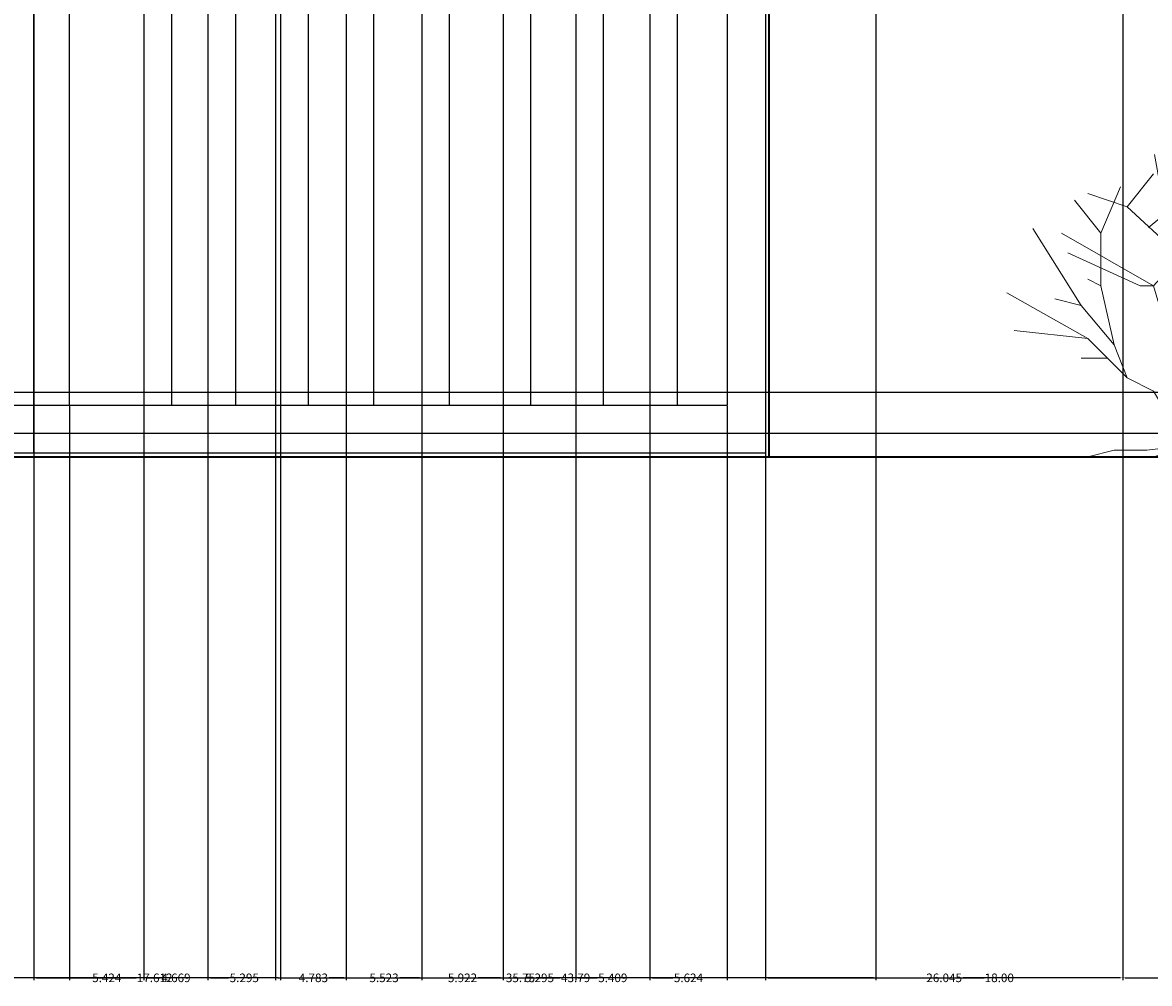
# Model space of a CAD drawing. Units: inches. Extents: x -13 to 809, y 112 to 656.
# Tile 11 of 55: x 257 to 339, y 112 to 182. Entities that reach past the tile are written whole.
import ezdxf

# ---------------------------------------------------------------- set-up
doc = ezdxf.new("R2010")
doc.units = ezdxf.units.IN
doc.header["$MEASUREMENT"] = 0
for name, color, linetype, lineweight in [('A-ANNO-DIMS', 2, 'Continuous', 18), ('A-DOOR', 4, 'Continuous', 25), ('A-ELEV', 7, 'Continuous', 35), ('L-PLNT', 3, 'Continuous', 18)]:
    doc.layers.add(name, color=color, linetype=linetype, lineweight=lineweight)
doc.styles.get("Standard").update_dxf_attribs({"font": 'arial.ttf'})
doc.dimstyles.get("Standard").update_dxf_attribs({"dimtxt": 0.625, "dimasz": 0.18, "dimexe": 0.18, "dimexo": 0.0625, "dimgap": 0.09, "dimtad": 0, "dimtih": 1, "dimtoh": 1, "dimdec": 4, "dimzin": 0, "dimdsep": 46, "dimlunit": 4, "dimtxsty": 'Standard', "dimcen": 0.09, "dimadec": 0, "dimazin": 0, "dimtfac": 1, "dimtdec": 4, "dimtofl": 0, "dimtmove": 0, "dimatfit": 3, "dimfxl": 1, "dimtolj": 1, "dimtzin": 0, "dimarcsym": 0})

# ---------------------------------------------------------------- blocks, each defined once
blk = doc.blocks.new('Shrub - elevation')
for p, q in [((-11.433, 18.289), (-10.457, 22.749)), ((-9.48, 19.775), (-8.992, 22.592)), ((-12.471, 19.775), (-12.898, 22.044)), ((-8.16, 17.76), (-10.56, 21.6)), ((-5.28, 19.2), (-3.84, 21.6)), ((-3.377, 18.602), (-2.888, 21.575)), ((-0.508, 21.888), (-0.081, 20.558)), ((0.041, 20.714), (1.384, 22.044)), ((0.102, 21.34), (0.835, 21.888)), ((-14.88, 18.24), (-12.96, 20.64)), ((-11.28, 19.619), (-12.104, 21.184)), ((-7.2, 19.68), (-6.24, 21.12)), ((-5.086, 17.741), (-5.513, 21.34)), ((-3.84, 16.8), (-0.96, 20.64)), ((-0.203, 19.149), (0.102, 21.34)), ((-0.02, 20.01), (0.896, 21.105)), ((-11.677, 19.071), (-12.471, 19.775)), ((-11.921, 18.836), (-10.64, 20.401)), ((-7.2, 19.68), (-8.64, 20.16)), ((-2.88, 15.84), (-2.4, 20.16)), ((-0.142, 19.384), (0.59, 20.401)), ((-14.88, 18.24), (-17.76, 19.2)), ((-16.8, 16.32), (-15.36, 19.68)), ((-10.579, 18.054), (-9.846, 19.697)), ((-8.16, 17.76), (-5.28, 19.2)), ((-4.8, 16.32), (-7.2, 19.68)), ((-2.88, 12.96), (-4.32, 19.68)), ((0.346, 13.203), (-0.203, 19.149)), ((-16.8, 16.32), (-18.72, 18.72)), ((-8.16, 12), (-14.88, 18.24)), ((-13.325, 16.724), (-11.433, 18.289)), ((-12.043, 15.628), (-11.921, 18.836)), ((-2.766, 16.802), (-3.377, 18.602)), ((1.323, 16.254), (3.642, 18.289)), ((-12.96, 12.48), (-8.16, 17.76)), ((-11.982, 16.802), (-10.579, 18.054)), ((-3.377, 15.315), (-5.086, 17.819)), ((1.44, 15.36), (2.88, 17.28)), ((-18.24, 11.04), (-21.755, 16.655)), ((-7.2, 14.88), (-3.84, 16.8)), ((-12.96, 12.48), (-19.68, 16.32)), ((-16.8, 12.48), (-16.8, 16.32)), ((-0.96, 10.56), (-2.88, 15.84)), ((0.346, 13.203), (1.323, 16.254)), ((2.4, 15.36), (3.36, 16.32)), ((-13.92, 12.48), (-19.2, 14.88)), ((-7.68, 12.48), (-7.2, 14.88)), ((0.96, 12), (1.44, 15.36)), ((0.96, 12), (2.88, 14.88)), ((1.92, 13.44), (2.4, 15.36)), ((-0.48, 10.8), (0.346, 13.203)), ((-16.8, 12.48), (-17.76, 12.96)), ((-15.84, 8.16), (-16.8, 12.48)), ((-12.96, 12.48), (-13.92, 12.48)), ((-10.56, 4.32), (-12.96, 12.48)), ((-6.72, 8.64), (-7.68, 12.48)), ((-3.36, 5.28), (-2.88, 12.96)), ((-17.76, 8.64), (-23.663, 11.961)), ((-18.24, 11.04), (-20.16, 11.52)), ((-8.64, 7.68), (-8.16, 12)), ((-1.92, 9.6), (0.96, 12)), ((-15.84, 8.16), (-18.24, 11.04)), ((-17.76, 8.64), (-23.128, 9.222)), ((-4.32, 2.88), (-1.92, 9.6)), ((-14.88, 5.76), (-17.76, 8.64)), ((-5.76, 5.28), (-6.72, 8.64)), ((-14.88, 5.76), (-15.84, 8.16)), ((-10.56, 4.32), (-8.64, 7.68)), ((-16.32, 7.2), (-18.24, 7.2)), ((-12.96, 4.8), (-14.88, 5.76)), ((-6.24, 2.88), (-5.76, 5.28)), ((-11.52, 2.4), (-12.96, 4.8)), ((-8.64, 1.92), (-10.56, 4.32)), ((-8.64, 0.96), (-4.32, 2.88)), ((-8.64, 0.96), (-6.24, 2.88)), ((-8.64, 0.96), (-11.52, 2.4)), ((-8.64, 0.96), (-8.64, 1.92)), ((-9.6, 0.96), (-13.44, 0.48)), ((-9.6, 0.96), (-12.96, 0)), ((-9.6, 0.96), (-7.68, 0.96)), ((-8.64, 0.96), (-2.88, 0.96)), ((-7.68, 0.96), (-6.24, 0.48)), ((-2.88, 0.96), (0, 0)), ((-15.84, 0.48), (-17.76, 0)), ((-13.44, 0.48), (-15.84, 0.48)), ((-6.24, 0.48), (-3.36, 0))]:
    blk.add_line(p, q)
blk = doc.blocks.new('*D15')
at = {"layer": 'A-ANNO-DIMS', "color": 0, "lineweight": -2, "transparency": 16777216}
for p, q in [((210.079, 223.038), (210.079, 112.34)), ((258.102, 210.722), (258.102, 112.34)), ((210.259, 112.52), (232.937, 112.52)), ((257.922, 112.52), (235.245, 112.52))]:
    blk.add_line(p, q, dxfattribs=at)
at = {"layer": 'A-ANNO-DIMS', "color": 0, "transparency": 16777216}
for points in [[(210.259, 112.55), (210.259, 112.49), (210.079, 112.52)], [(257.922, 112.55), (257.922, 112.49), (258.102, 112.52)]]:
    blk.add_solid(points, dxfattribs=at)
at = {"layer": 'Defpoints', "color": 0, "transparency": 16777216}
for p in [(210.079, 223.1), (258.102, 210.785), (258.102, 112.52)]:
    blk.add_point(p, dxfattribs=at)
at = {"layer": 'A-ANNO-DIMS', "color": 0, "transparency": 16777216, "insert": (234.091, 112.52), "char_height": 0.625, "attachment_point": 5}
blk.add_mtext('\\A1;48.02', dxfattribs=at)
blk = doc.blocks.new('*D16')
at = {"layer": 'A-ANNO-DIMS', "color": 0, "lineweight": -2, "transparency": 16777216}
for p, q in [((275.715, 223.038), (275.715, 112.34)), ((258.102, 210.722), (258.102, 112.34)), ((258.282, 112.52), (265.554, 112.52)), ((275.535, 112.52), (268.263, 112.52))]:
    blk.add_line(p, q, dxfattribs=at)
at = {"layer": 'A-ANNO-DIMS', "color": 0, "transparency": 16777216}
for points in [[(258.282, 112.55), (258.282, 112.49), (258.102, 112.52)], [(275.535, 112.55), (275.535, 112.49), (275.715, 112.52)]]:
    blk.add_solid(points, dxfattribs=at)
at = {"layer": 'Defpoints', "color": 0, "transparency": 16777216}
for p in [(275.715, 223.1), (258.102, 210.785), (275.715, 112.52)]:
    blk.add_point(p, dxfattribs=at)
at = {"layer": 'A-ANNO-DIMS', "color": 0, "transparency": 16777216, "insert": (266.908, 112.52), "char_height": 0.625, "attachment_point": 5}
blk.add_mtext('\\A1;17.612', dxfattribs=at)
blk = doc.blocks.new('*D17')
at = {"layer": 'A-ANNO-DIMS', "color": 0, "lineweight": -2, "transparency": 16777216}
for p, q in [((275.715, 223.038), (275.715, 112.34)), ((311.463, 210.722), (311.463, 112.34)), ((275.895, 112.52), (292.442, 112.52)), ((311.283, 112.52), (294.735, 112.52))]:
    blk.add_line(p, q, dxfattribs=at)
at = {"layer": 'A-ANNO-DIMS', "color": 0, "transparency": 16777216}
for points in [[(275.895, 112.55), (275.895, 112.49), (275.715, 112.52)], [(311.283, 112.55), (311.283, 112.49), (311.463, 112.52)]]:
    blk.add_solid(points, dxfattribs=at)
at = {"layer": 'Defpoints', "color": 0, "transparency": 16777216}
for p in [(275.715, 223.1), (311.463, 210.785), (311.463, 112.52)]:
    blk.add_point(p, dxfattribs=at)
at = {"layer": 'A-ANNO-DIMS', "color": 0, "transparency": 16777216, "insert": (293.589, 112.52), "char_height": 0.625, "attachment_point": 5}
blk.add_mtext('\\A1;35.75', dxfattribs=at)
blk = doc.blocks.new('*D18')
at = {"layer": 'A-ANNO-DIMS', "color": 0, "lineweight": -2, "transparency": 16777216}
for p, q in [((337.507, 306.457), (337.507, 112.34)), ((311.463, 210.722), (311.463, 112.34)), ((311.643, 112.52), (323.09, 112.52)), ((337.327, 112.52), (325.88, 112.52))]:
    blk.add_line(p, q, dxfattribs=at)
at = {"layer": 'A-ANNO-DIMS', "color": 0, "transparency": 16777216}
for points in [[(311.643, 112.55), (311.643, 112.49), (311.463, 112.52)], [(337.327, 112.55), (337.327, 112.49), (337.507, 112.52)]]:
    blk.add_solid(points, dxfattribs=at)
at = {"layer": 'Defpoints', "color": 0, "transparency": 16777216}
for p in [(337.507, 306.52), (311.463, 210.785), (337.507, 112.52)]:
    blk.add_point(p, dxfattribs=at)
at = {"layer": 'A-ANNO-DIMS', "color": 0, "transparency": 16777216, "insert": (324.485, 112.52), "char_height": 0.625, "attachment_point": 5}
blk.add_mtext('\\A1;26.045', dxfattribs=at)
blk = doc.blocks.new('*D19')
at = {"layer": 'A-ANNO-DIMS', "color": 0, "lineweight": -2, "transparency": 16777216}
for p, q in [((337.507, 306.457), (337.507, 112.34)), ((365.938, 210.722), (365.938, 112.34)), ((337.687, 112.52), (350.573, 112.52)), ((365.758, 112.52), (352.873, 112.52))]:
    blk.add_line(p, q, dxfattribs=at)
at = {"layer": 'A-ANNO-DIMS', "color": 0, "transparency": 16777216}
for points in [[(337.687, 112.55), (337.687, 112.49), (337.507, 112.52)], [(365.758, 112.55), (365.758, 112.49), (365.938, 112.52)]]:
    blk.add_solid(points, dxfattribs=at)
at = {"layer": 'Defpoints', "color": 0, "transparency": 16777216}
for p in [(337.507, 306.52), (365.938, 210.785), (365.938, 112.52)]:
    blk.add_point(p, dxfattribs=at)
at = {"layer": 'A-ANNO-DIMS', "color": 0, "transparency": 16777216, "insert": (351.723, 112.52), "char_height": 0.625, "attachment_point": 5}
blk.add_mtext('\\A1;28.43', dxfattribs=at)
blk = doc.blocks.new('*D108')
at = {"layer": 'A-ANNO-DIMS', "color": 0, "lineweight": -2, "transparency": 16777216}
for p, q in [((319.507, 324.457), (319.507, 112.34)), ((337.507, 306.457), (337.507, 112.34)), ((319.687, 112.52), (327.393, 112.52)), ((337.327, 112.52), (329.621, 112.52))]:
    blk.add_line(p, q, dxfattribs=at)
at = {"layer": 'A-ANNO-DIMS', "color": 0, "transparency": 16777216}
for points in [[(319.687, 112.55), (319.687, 112.49), (319.507, 112.52)], [(337.327, 112.55), (337.327, 112.49), (337.507, 112.52)]]:
    blk.add_solid(points, dxfattribs=at)
at = {"layer": 'Defpoints', "color": 0, "transparency": 16777216}
for p in [(319.507, 324.52), (337.507, 306.52), (337.507, 112.52)]:
    blk.add_point(p, dxfattribs=at)
at = {"layer": 'A-ANNO-DIMS', "color": 0, "transparency": 16777216, "insert": (328.507, 112.52), "char_height": 0.625, "attachment_point": 5}
blk.add_mtext('\\A1;18.00', dxfattribs=at)
blk = doc.blocks.new('*D112')
at = {"layer": 'A-ANNO-DIMS', "color": 0, "lineweight": -2, "transparency": 16777216}
for p, q in [((210.079, 361.229), (210.079, 112.34)), ((275.715, 361.229), (275.715, 112.34)), ((210.259, 112.52), (241.752, 112.52)), ((275.535, 112.52), (244.042, 112.52))]:
    blk.add_line(p, q, dxfattribs=at)
at = {"layer": 'A-ANNO-DIMS', "color": 0, "transparency": 16777216}
for points in [[(210.259, 112.55), (210.259, 112.49), (210.079, 112.52)], [(275.535, 112.55), (275.535, 112.49), (275.715, 112.52)]]:
    blk.add_solid(points, dxfattribs=at)
at = {"layer": 'Defpoints', "color": 0, "transparency": 16777216}
for p in [(210.079, 361.292), (275.715, 361.292), (275.715, 112.52)]:
    blk.add_point(p, dxfattribs=at)
at = {"layer": 'A-ANNO-DIMS', "color": 0, "transparency": 16777216, "insert": (242.897, 112.52), "char_height": 0.625, "attachment_point": 5}
blk.add_mtext('\\A1;65.64', dxfattribs=at)
blk = doc.blocks.new('*D113')
at = {"layer": 'A-ANNO-DIMS', "color": 0, "lineweight": -2, "transparency": 16777216}
for p, q in [((275.715, 361.229), (275.715, 112.34)), ((319.507, 324.457), (319.507, 112.34)), ((275.895, 112.52), (296.453, 112.52)), ((319.327, 112.52), (298.769, 112.52))]:
    blk.add_line(p, q, dxfattribs=at)
at = {"layer": 'A-ANNO-DIMS', "color": 0, "transparency": 16777216}
for points in [[(275.895, 112.55), (275.895, 112.49), (275.715, 112.52)], [(319.327, 112.55), (319.327, 112.49), (319.507, 112.52)]]:
    blk.add_solid(points, dxfattribs=at)
at = {"layer": 'Defpoints', "color": 0, "transparency": 16777216}
for p in [(275.715, 361.292), (319.507, 324.52), (319.507, 112.52)]:
    blk.add_point(p, dxfattribs=at)
at = {"layer": 'A-ANNO-DIMS', "color": 0, "transparency": 16777216, "insert": (297.611, 112.52), "char_height": 0.625, "attachment_point": 5}
blk.add_mtext('\\A1;43.79', dxfattribs=at)
blk = doc.blocks.new('*D115')
at = {"layer": 'A-ANNO-DIMS', "color": 0, "lineweight": -2, "transparency": 16777216}
for p, q in [((311.4, 210.785), (-12.099, 210.785)), ((-11.919, 210.605), (-11.919, 181.062)), ((-11.919, 150.7), (-11.919, 180.243)), ((311.637, 150.52), (-12.099, 150.52))]:
    blk.add_line(p, q, dxfattribs=at)
at = {"layer": 'A-ANNO-DIMS', "color": 0, "transparency": 16777216}
for points in [[(-11.949, 210.605), (-11.889, 210.605), (-11.919, 210.785)], [(-11.949, 150.7), (-11.889, 150.7), (-11.919, 150.52)]]:
    blk.add_solid(points, dxfattribs=at)
at = {"layer": 'Defpoints', "color": 0, "transparency": 16777216}
for p in [(-11.919, 210.785), (311.463, 210.785), (311.699, 150.52)]:
    blk.add_point(p, dxfattribs=at)
at = {"layer": 'A-ANNO-DIMS', "color": 0, "transparency": 16777216, "insert": (-11.919, 180.652), "char_height": 0.625, "attachment_point": 5}
blk.add_mtext('\\A1;60.27', dxfattribs=at)
blk = doc.blocks.new('*D117')
at = {"layer": 'A-ANNO-DIMS', "color": 0, "lineweight": -2, "transparency": 16777216}
for p, q in [((260.642, 154.272), (-12.099, 154.272)), ((-11.919, 154.092), (-11.919, 152.938)), ((-11.919, 150.965), (-11.919, 152.119)), ((258.04, 150.785), (-12.099, 150.785))]:
    blk.add_line(p, q, dxfattribs=at)
at = {"layer": 'A-ANNO-DIMS', "color": 0, "transparency": 16777216}
for points in [[(-11.949, 154.092), (-11.889, 154.092), (-11.919, 154.272)], [(-11.949, 150.965), (-11.889, 150.965), (-11.919, 150.785)]]:
    blk.add_solid(points, dxfattribs=at)
at = {"layer": 'Defpoints', "color": 0, "transparency": 16777216}
for p in [(260.705, 154.272), (-11.919, 150.785), (258.102, 150.785)]:
    blk.add_point(p, dxfattribs=at)
at = {"layer": 'A-ANNO-DIMS', "color": 0, "transparency": 16777216, "insert": (-11.919, 152.529), "char_height": 0.625, "attachment_point": 5}
blk.add_mtext('\\A1;3.487', dxfattribs=at)
blk = doc.blocks.new('*D120')
at = {"layer": 'A-ANNO-DIMS', "color": 0, "lineweight": -2, "transparency": 16777216}
for p, q in [((260.705, 154.21), (260.705, 112.34)), ((266.129, 154.21), (266.129, 112.34)), ((260.885, 112.52), (262.273, 112.52)), ((265.949, 112.52), (264.56, 112.52))]:
    blk.add_line(p, q, dxfattribs=at)
at = {"layer": 'A-ANNO-DIMS', "color": 0, "transparency": 16777216}
for points in [[(260.885, 112.55), (260.885, 112.49), (260.705, 112.52)], [(265.949, 112.55), (265.949, 112.49), (266.129, 112.52)]]:
    blk.add_solid(points, dxfattribs=at)
at = {"layer": 'Defpoints', "color": 0, "transparency": 16777216}
for p in [(260.705, 154.272), (266.129, 154.272), (266.129, 112.52)]:
    blk.add_point(p, dxfattribs=at)
at = {"layer": 'A-ANNO-DIMS', "color": 0, "transparency": 16777216, "insert": (263.417, 112.52), "char_height": 0.625, "attachment_point": 5}
blk.add_mtext('\\A1;5.424', dxfattribs=at)
blk = doc.blocks.new('*D121')
at = {"layer": 'A-ANNO-DIMS', "color": 0, "lineweight": -2, "transparency": 16777216}
for p, q in [((266.129, 154.21), (266.129, 112.34)), ((270.798, 154.21), (270.798, 112.34)), ((266.309, 112.52), (267.305, 112.52)), ((270.618, 112.52), (269.621, 112.52))]:
    blk.add_line(p, q, dxfattribs=at)
at = {"layer": 'A-ANNO-DIMS', "color": 0, "transparency": 16777216}
for points in [[(266.309, 112.55), (266.309, 112.49), (266.129, 112.52)], [(270.618, 112.55), (270.618, 112.49), (270.798, 112.52)]]:
    blk.add_solid(points, dxfattribs=at)
at = {"layer": 'Defpoints', "color": 0, "transparency": 16777216}
for p in [(266.129, 154.272), (270.798, 154.272), (270.798, 112.52)]:
    blk.add_point(p, dxfattribs=at)
at = {"layer": 'A-ANNO-DIMS', "color": 0, "transparency": 16777216, "insert": (268.463, 112.52), "char_height": 0.625, "attachment_point": 5}
blk.add_mtext('\\A1;4.669', dxfattribs=at)
blk = doc.blocks.new('*D122')
at = {"layer": 'A-ANNO-DIMS', "color": 0, "lineweight": -2, "transparency": 16777216}
for p, q in [((270.798, 154.21), (270.798, 112.34)), ((276.093, 154.21), (276.093, 112.34)), ((270.978, 112.52), (272.298, 112.52)), ((275.913, 112.52), (274.592, 112.52))]:
    blk.add_line(p, q, dxfattribs=at)
at = {"layer": 'A-ANNO-DIMS', "color": 0, "transparency": 16777216}
for points in [[(270.978, 112.55), (270.978, 112.49), (270.798, 112.52)], [(275.913, 112.55), (275.913, 112.49), (276.093, 112.52)]]:
    blk.add_solid(points, dxfattribs=at)
at = {"layer": 'Defpoints', "color": 0, "transparency": 16777216}
for p in [(270.798, 154.272), (276.093, 154.272), (276.093, 112.52)]:
    blk.add_point(p, dxfattribs=at)
at = {"layer": 'A-ANNO-DIMS', "color": 0, "transparency": 16777216, "insert": (273.445, 112.52), "char_height": 0.625, "attachment_point": 5}
blk.add_mtext('\\A1;5.295', dxfattribs=at)
blk = doc.blocks.new('*D123')
at = {"layer": 'A-ANNO-DIMS', "color": 0, "lineweight": -2, "transparency": 16777216}
for p, q in [((276.093, 154.21), (276.093, 112.34)), ((280.875, 154.21), (280.875, 112.34)), ((276.273, 112.52), (277.327, 112.52)), ((280.695, 112.52), (279.641, 112.52))]:
    blk.add_line(p, q, dxfattribs=at)
at = {"layer": 'A-ANNO-DIMS', "color": 0, "transparency": 16777216}
for points in [[(276.273, 112.55), (276.273, 112.49), (276.093, 112.52)], [(280.695, 112.55), (280.695, 112.49), (280.875, 112.52)]]:
    blk.add_solid(points, dxfattribs=at)
at = {"layer": 'Defpoints', "color": 0, "transparency": 16777216}
for p in [(276.093, 154.272), (280.875, 154.272), (280.875, 112.52)]:
    blk.add_point(p, dxfattribs=at)
at = {"layer": 'A-ANNO-DIMS', "color": 0, "transparency": 16777216, "insert": (278.484, 112.52), "char_height": 0.625, "attachment_point": 5}
blk.add_mtext('\\A1;4.783', dxfattribs=at)
blk = doc.blocks.new('*D124')
at = {"layer": 'A-ANNO-DIMS', "color": 0, "lineweight": -2, "transparency": 16777216}
for p, q in [((280.875, 154.21), (280.875, 112.34)), ((286.398, 154.21), (286.398, 112.34)), ((281.055, 112.52), (282.492, 112.52)), ((286.218, 112.52), (284.782, 112.52))]:
    blk.add_line(p, q, dxfattribs=at)
at = {"layer": 'A-ANNO-DIMS', "color": 0, "transparency": 16777216}
for points in [[(281.055, 112.55), (281.055, 112.49), (280.875, 112.52)], [(286.218, 112.55), (286.218, 112.49), (286.398, 112.52)]]:
    blk.add_solid(points, dxfattribs=at)
at = {"layer": 'Defpoints', "color": 0, "transparency": 16777216}
for p in [(280.875, 154.272), (286.398, 154.272), (286.398, 112.52)]:
    blk.add_point(p, dxfattribs=at)
at = {"layer": 'A-ANNO-DIMS', "color": 0, "transparency": 16777216, "insert": (283.637, 112.52), "char_height": 0.625, "attachment_point": 5}
blk.add_mtext('\\A1;5.523', dxfattribs=at)
blk = doc.blocks.new('*D125')
at = {"layer": 'A-ANNO-DIMS', "color": 0, "lineweight": -2, "transparency": 16777216}
for p, q in [((286.398, 154.21), (286.398, 112.34)), ((292.32, 154.21), (292.32, 112.34)), ((286.578, 112.52), (288.218, 112.52)), ((292.14, 112.52), (290.501, 112.52))]:
    blk.add_line(p, q, dxfattribs=at)
at = {"layer": 'A-ANNO-DIMS', "color": 0, "transparency": 16777216}
for points in [[(286.578, 112.55), (286.578, 112.49), (286.398, 112.52)], [(292.14, 112.55), (292.14, 112.49), (292.32, 112.52)]]:
    blk.add_solid(points, dxfattribs=at)
at = {"layer": 'Defpoints', "color": 0, "transparency": 16777216}
for p in [(286.398, 154.272), (292.32, 154.272), (292.32, 112.52)]:
    blk.add_point(p, dxfattribs=at)
at = {"layer": 'A-ANNO-DIMS', "color": 0, "transparency": 16777216, "insert": (289.359, 112.52), "char_height": 0.625, "attachment_point": 5}
blk.add_mtext('\\A1;5.922', dxfattribs=at)
blk = doc.blocks.new('*D126')
at = {"layer": 'A-ANNO-DIMS', "color": 0, "lineweight": -2, "transparency": 16777216}
for p, q in [((292.32, 154.21), (292.32, 112.34)), ((297.615, 154.21), (297.615, 112.34)), ((292.5, 112.52), (293.821, 112.52)), ((297.435, 112.52), (296.114, 112.52))]:
    blk.add_line(p, q, dxfattribs=at)
at = {"layer": 'A-ANNO-DIMS', "color": 0, "transparency": 16777216}
for points in [[(292.5, 112.55), (292.5, 112.49), (292.32, 112.52)], [(297.435, 112.55), (297.435, 112.49), (297.615, 112.52)]]:
    blk.add_solid(points, dxfattribs=at)
at = {"layer": 'Defpoints', "color": 0, "transparency": 16777216}
for p in [(292.32, 154.272), (297.615, 154.272), (297.615, 112.52)]:
    blk.add_point(p, dxfattribs=at)
at = {"layer": 'A-ANNO-DIMS', "color": 0, "transparency": 16777216, "insert": (294.968, 112.52), "char_height": 0.625, "attachment_point": 5}
blk.add_mtext('\\A1;5.295', dxfattribs=at)
blk = doc.blocks.new('*D127')
at = {"layer": 'A-ANNO-DIMS', "color": 0, "lineweight": -2, "transparency": 16777216}
for p, q in [((297.615, 154.21), (297.615, 112.34)), ((303.024, 154.21), (303.024, 112.34)), ((297.795, 112.52), (299.175, 112.52)), ((302.844, 112.52), (301.465, 112.52))]:
    blk.add_line(p, q, dxfattribs=at)
at = {"layer": 'A-ANNO-DIMS', "color": 0, "transparency": 16777216}
for points in [[(297.795, 112.55), (297.795, 112.49), (297.615, 112.52)], [(302.844, 112.55), (302.844, 112.49), (303.024, 112.52)]]:
    blk.add_solid(points, dxfattribs=at)
at = {"layer": 'Defpoints', "color": 0, "transparency": 16777216}
for p in [(297.615, 154.272), (303.024, 154.272), (303.024, 112.52)]:
    blk.add_point(p, dxfattribs=at)
at = {"layer": 'A-ANNO-DIMS', "color": 0, "transparency": 16777216, "insert": (300.32, 112.52), "char_height": 0.625, "attachment_point": 5}
blk.add_mtext('\\A1;5.409', dxfattribs=at)
blk = doc.blocks.new('*D128')
at = {"layer": 'A-ANNO-DIMS', "color": 0, "lineweight": -2, "transparency": 16777216}
for p, q in [((303.024, 154.21), (303.024, 112.34)), ((308.649, 154.21), (308.649, 112.34)), ((303.204, 112.52), (304.693, 112.52)), ((308.469, 112.52), (306.98, 112.52))]:
    blk.add_line(p, q, dxfattribs=at)
at = {"layer": 'A-ANNO-DIMS', "color": 0, "transparency": 16777216}
for points in [[(303.204, 112.55), (303.204, 112.49), (303.024, 112.52)], [(308.469, 112.55), (308.469, 112.49), (308.649, 112.52)]]:
    blk.add_solid(points, dxfattribs=at)
at = {"layer": 'Defpoints', "color": 0, "transparency": 16777216}
for p in [(303.024, 154.272), (308.649, 154.272), (308.649, 112.52)]:
    blk.add_point(p, dxfattribs=at)
at = {"layer": 'A-ANNO-DIMS', "color": 0, "transparency": 16777216, "insert": (305.837, 112.52), "char_height": 0.625, "attachment_point": 5}
blk.add_mtext('\\A1;5.624', dxfattribs=at)
blk = doc.blocks.new('*D131')
at = {"layer": 'A-ANNO-DIMS', "color": 0, "lineweight": -2, "transparency": 16777216}
for p, q in [((368.876, 155.214), (-12.099, 155.214)), ((-11.919, 155.034), (-11.919, 154.123)), ((-11.919, 152.394), (-11.919, 153.305)), ((365.876, 152.214), (-12.099, 152.214))]:
    blk.add_line(p, q, dxfattribs=at)
at = {"layer": 'A-ANNO-DIMS', "color": 0, "transparency": 16777216}
for points in [[(-11.949, 155.034), (-11.889, 155.034), (-11.919, 155.214)], [(-11.949, 152.394), (-11.889, 152.394), (-11.919, 152.214)]]:
    blk.add_solid(points, dxfattribs=at)
at = {"layer": 'Defpoints', "color": 0, "transparency": 16777216}
for p in [(368.938, 155.214), (-11.919, 152.214), (365.938, 152.214)]:
    blk.add_point(p, dxfattribs=at)
at = {"layer": 'A-ANNO-DIMS', "color": 0, "transparency": 16777216, "insert": (-11.919, 153.714), "char_height": 0.625, "attachment_point": 5}
blk.add_mtext('\\A1;3.00', dxfattribs=at)

msp = doc.modelspace()

# ---------------------------------------------------------------- linework, layer by layer
at = {"layer": 'A-DOOR'}
for p, q in [((266.1286, 207.3724), (266.1286, 154.2723)), ((268.1286, 207.3724), (268.1286, 154.2723)), ((270.7975, 207.3724), (270.7975, 154.2723)), ((272.7975, 207.3724), (272.7975, 154.2723)), ((276.0927, 207.3724), (276.0927, 154.2723)), ((278.0927, 207.3724), (278.0927, 154.2723)), ((280.8755, 207.3724), (280.8755, 154.2723)), ((282.8755, 207.3724), (282.8755, 154.2723)), ((286.3985, 207.3724), (286.3985, 154.2723)), ((288.3985, 207.3724), (288.3985, 154.2723)), ((292.32, 207.3724), (292.32, 154.2723)), ((294.32, 207.3724), (294.32, 154.2723)), ((297.6152, 207.3724), (297.6152, 154.2723)), ((299.6152, 207.3724), (299.6152, 154.2723)), ((303.0243, 207.3724), (303.0243, 154.2723)), ((305.0243, 207.3724), (305.0243, 154.2723))]:
    msp.add_line(p, q, dxfattribs=at)
for points in [[(258.1022, 210.7849), (311.4627, 210.7849), (311.4627, 150.7849), (258.1022, 150.7849)], [(260.7048, 207.3724), (308.6488, 207.3724), (308.6488, 154.2723), (260.7048, 154.2723)]]:
    msp.add_lwpolyline(points, close=True, dxfattribs=at)
at = {"layer": 'A-ELEV'}
for p, q in [((311.6991, 210.4452), (311.6991, 150.5199)), ((109.5888, 150.5199), (649.5888, 150.5199))]:
    msp.add_line(p, q, dxfattribs=at)

# ---------------------------------------------------------------- block references
at = {"layer": 'L-PLNT'}
msp.add_blockref('Shrub - elevation', (352.7114, 150.5199), dxfattribs=at)

# ---------------------------------------------------------------- dimensions: what is measured, and where the dimension line sits
at = {"layer": 'A-ANNO-DIMS'}
for base, p1, p2, override, picture, middle in [((275.7145, 112.5199), (210.0791, 361.2915), (275.7145, 361.2915), {"dimdec": 2, "dimlfac": 1, "dimrnd": 0, "dimzin": 0, "dimdsep": 46, "dimlunit": 2}, '*D112', (242.8968, 112.5199)), ((319.5074, 112.5199), (275.7145, 361.2915), (319.5074, 324.5199), {"dimdec": 2, "dimlfac": 1, "dimrnd": 0, "dimzin": 0, "dimdsep": 46, "dimlunit": 2}, '*D113', (297.611, 112.5199)), ((337.5074, 112.5199), (319.5074, 324.5199), (337.5074, 306.5199), {"dimdec": 2, "dimlfac": 1, "dimrnd": 0, "dimzin": 0, "dimdsep": 46, "dimlunit": 2}, '*D108', (328.5074, 112.5199)), ((337.5074, 112.5199), (311.4627, 210.7849), (337.5074, 306.5199), {"dimdec": 3, "dimlfac": 1, "dimrnd": 0, "dimzin": 0, "dimdsep": 46, "dimlunit": 2}, '*D18', (324.4851, 112.5199)), ((365.9383, 112.5199), (337.5074, 306.5199), (365.9383, 210.7849), {"dimdec": 2, "dimlfac": 1, "dimrnd": 0, "dimzin": 0, "dimdsep": 46, "dimlunit": 2}, '*D19', (351.7228, 112.5199)), ((258.1022, 112.5199), (210.0791, 223.1), (258.1022, 210.7849), {"dimdec": 2, "dimlfac": 1, "dimrnd": 0, "dimzin": 0, "dimdsep": 46, "dimlunit": 2}, '*D15', (234.0906, 112.5199)), ((275.7145, 112.5199), (258.1022, 210.7849), (275.7145, 223.1), {"dimdec": 3, "dimlfac": 1, "dimrnd": 0, "dimzin": 0, "dimdsep": 46, "dimlunit": 2}, '*D16', (266.9083, 112.5199)), ((311.4627, 112.5199), (275.7145, 223.1), (311.4627, 210.7849), {"dimdec": 2, "dimlfac": 1, "dimrnd": 0, "dimzin": 0, "dimdsep": 46, "dimlunit": 2}, '*D17', (293.5886, 112.5199)), ((266.1286, 112.5199), (260.7048, 154.2723), (266.1286, 154.2723), {"dimdec": 3, "dimlfac": 1, "dimrnd": 0, "dimzin": 0, "dimdsep": 46, "dimlunit": 2}, '*D120', (263.4167, 112.5199)), ((270.7975, 112.5199), (266.1286, 154.2723), (270.7975, 154.2723), {"dimdec": 3, "dimlfac": 1, "dimrnd": 0, "dimzin": 0, "dimdsep": 46, "dimlunit": 2}, '*D121', (268.4631, 112.5199)), ((276.0927, 112.5199), (270.7975, 154.2723), (276.0927, 154.2723), {"dimdec": 3, "dimlfac": 1, "dimrnd": 0, "dimzin": 0, "dimdsep": 46, "dimlunit": 2}, '*D122', (273.4451, 112.5199)), ((280.8755, 112.5199), (276.0927, 154.2723), (280.8755, 154.2723), {"dimdec": 3, "dimlfac": 1, "dimrnd": 0, "dimzin": 0, "dimdsep": 46, "dimlunit": 2}, '*D123', (278.4841, 112.5199)), ((286.3985, 112.5199), (280.8755, 154.2723), (286.3985, 154.2723), {"dimdec": 3, "dimlfac": 1, "dimrnd": 0, "dimzin": 0, "dimdsep": 46, "dimlunit": 2}, '*D124', (283.637, 112.5199)), ((292.32, 112.51989), (286.39847, 154.27226), (292.32, 154.27226), {"dimdec": 3, "dimlfac": 1, "dimrnd": 0, "dimzin": 0, "dimdsep": 46, "dimlunit": 2}, '*D125', (289.35924, 112.51989)), ((297.6152, 112.5199), (292.32, 154.2723), (297.6152, 154.2723), {"dimdec": 3, "dimlfac": 1, "dimrnd": 0, "dimzin": 0, "dimdsep": 46, "dimlunit": 2}, '*D126', (294.9676, 112.5199)), ((303.0243, 112.5199), (297.6152, 154.2723), (303.0243, 154.2723), {"dimdec": 3, "dimlfac": 1, "dimrnd": 0, "dimzin": 0, "dimdsep": 46, "dimlunit": 2}, '*D127', (300.3198, 112.5199)), ((308.64878, 112.51989), (303.02432, 154.27226), (308.64878, 154.27226), {"dimdec": 3, "dimlfac": 1, "dimrnd": 0, "dimzin": 0, "dimdsep": 46, "dimlunit": 2}, '*D128', (305.83655, 112.51989))]:
    dim = msp.add_linear_dim(base=base, p1=p1, p2=p2, dimstyle='Standard', override=override, dxfattribs=at)
    dim.commit()
    dim.dimension.update_dxf_attribs({"geometry": picture, "text_midpoint": middle})
for base, p1, p2, override, picture, middle in [((-11.91915, 210.78493), (311.6991, 150.51989), (311.46269, 210.78493), {"dimdec": 2, "dimlfac": 1, "dimrnd": 0, "dimzin": 0, "dimdsep": 46, "dimlunit": 2}, '*D115', (-11.91915, 180.65241)), ((-11.9191, 152.2141), (368.9383, 155.2141), (365.9383, 152.2141), {"dimdec": 2, "dimlfac": 1, "dimrnd": 0, "dimzin": 0, "dimdsep": 46, "dimlunit": 2}, '*D131', (-11.9191, 153.7141)), ((-11.9191, 150.7849), (260.7048, 154.2723), (258.1022, 150.7849), {"dimdec": 3, "dimlfac": 1, "dimrnd": 0, "dimzin": 0, "dimdsep": 46, "dimlunit": 2}, '*D117', (-11.9191, 152.5286))]:
    dim = msp.add_linear_dim(base=base, p1=p1, p2=p2, angle=90, dimstyle='Standard', override=override, dxfattribs=at)
    dim.commit()
    dim.dimension.update_dxf_attribs({"geometry": picture, "text_midpoint": middle})

doc.saveas('drawing.dxf')
